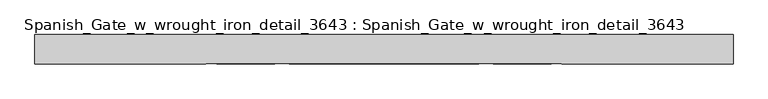
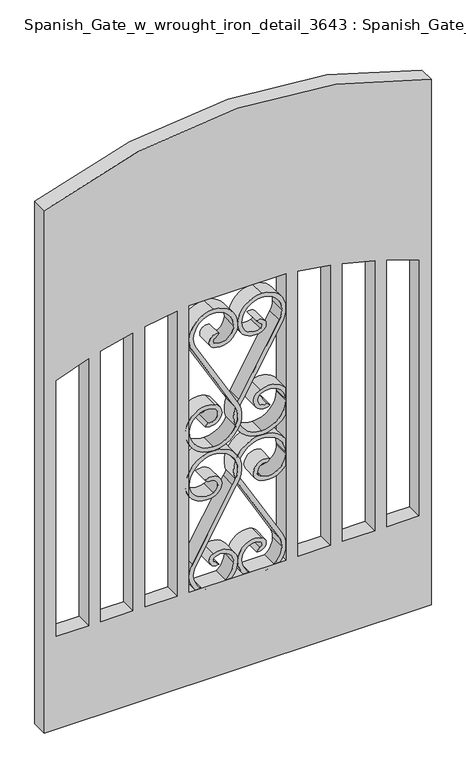
"""IFC4 building model written with IfcOpenShell, lengths in millimetres: proxy geometry, Spanish_Gate_w_wrought_iron_detail_3643 : Spanish_Gate_w_wrought_iron_detail_3643."""

from ifc_helpers import new_model, si_unit, point, frame, frame_2d, origin, place, context, project, spatial, polyline, circle_curve, trimmed, segment, composite_curve, outline, extrude, source, transform, mapped, element, save


def spanish_gate_w_wrought_iron_detail_3643_spanish_gate_w_2ba93c97(model_context):
    return source(origin(), model_context, "Body", "SweptSolid", [
        extrude(outline(composite_curve([segment(polyline([(-271.0336622, 609.6), (1477.5257324, 609.6)]), True, "CONTINUOUS"), segment(trimmed(circle_curve(frame_2d((13.3799195, 11.1413161)), 1581.7318856), [point((1477.5257324, 609.6))], [point((1468.218734, -609.6))], False, "CARTESIAN"), True, "CONTINUOUS"), segment(polyline([(1468.218734, -609.6), (-271.0336622, -609.6), (-271.0336622, 609.6)]), True, "CONTINUOUS")], self_intersect=False), holes=[composite_curve([segment(polyline([(38.1, -469.9), (38.1, -571.5), (888.7988681, -571.5)]), True, "CONTINUOUS"), segment(trimmed(circle_curve(frame_2d((-545.1422563, 0.0)), 1543.6318856), [point((888.7988681, -571.5))], [point((925.2295974, -469.9))], True, "CARTESIAN"), True, "CONTINUOUS"), segment(polyline([(925.2295974, -469.9), (38.1, -469.9)]), True, "CONTINUOUS")], self_intersect=False), composite_curve([segment(polyline([(38.1, 571.5), (38.1, 469.9), (925.2295974, 469.9)]), True, "CONTINUOUS"), segment(trimmed(circle_curve(frame_2d((-545.1422563, 0.0)), 1543.6318856), [point((925.2295974, 469.9))], [point((888.7988681, 571.5))], True, "CARTESIAN"), True, "CONTINUOUS"), segment(polyline([(888.7988681, 571.5), (38.1, 571.5)]), True, "CONTINUOUS")], self_intersect=False), composite_curve([segment(polyline([(38.1, -431.8), (936.8658942, -431.8)]), True, "CONTINUOUS"), segment(trimmed(circle_curve(frame_2d((-545.1422563, 0.0)), 1543.6318856), [point((936.8658942, -431.8))], [point((962.7593845, -330.2))], True, "CARTESIAN"), True, "CONTINUOUS"), segment(polyline([(962.7593845, -330.2), (38.1, -330.2), (38.1, -431.8)]), True, "CONTINUOUS")], self_intersect=False), composite_curve([segment(polyline([(936.8658942, 431.8), (38.1, 431.8), (38.1, 330.2), (962.7593845, 330.2)]), True, "CONTINUOUS"), segment(trimmed(circle_curve(frame_2d((-545.1422563, 0.0)), 1543.6318856), [point((962.7593845, 330.2))], [point((936.8658942, 431.8))], True, "CARTESIAN"), True, "CONTINUOUS")], self_intersect=False), composite_curve([segment(polyline([(38.1, -292.1), (970.6007919, -292.1)]), True, "CONTINUOUS"), segment(trimmed(circle_curve(frame_2d((-545.1422563, 0.0)), 1543.6318856), [point((970.6007919, -292.1))], [point((986.6897019, -190.5))], True, "CARTESIAN"), True, "CONTINUOUS"), segment(polyline([(986.6897019, -190.5), (38.1, -190.5), (38.1, -292.1)]), True, "CONTINUOUS")], self_intersect=False), composite_curve([segment(polyline([(970.6007919, 292.1), (38.1, 292.1), (38.1, 190.5), (986.6897019, 190.5)]), True, "CONTINUOUS"), segment(trimmed(circle_curve(frame_2d((-545.1422563, 0.0)), 1543.6318856), [point((986.6897019, 190.5))], [point((970.6007919, 292.1))], True, "CARTESIAN"), True, "CONTINUOUS")], self_intersect=False), composite_curve([segment(polyline([(38.1, 152.4), (38.1, -152.4), (990.9481181, -152.4)]), True, "CONTINUOUS"), segment(trimmed(circle_curve(frame_2d((-545.1422563, 0.0)), 1543.6318856), [point((990.9481181, -152.4))], [point((990.9481181, 152.4))], True, "CARTESIAN"), True, "CONTINUOUS"), segment(polyline([(990.9481181, 152.4), (38.1, 152.4)]), True, "CONTINUOUS")], self_intersect=False)]), frame((0.0, -50.8, 0.0), z_axis=(0.0, 1.0, 0.0), x_axis=(0.0, 0.0, 1.0)), (0.0, 0.0, 1.0), 50.8),
        extrude(outline(composite_curve([segment(trimmed(circle_curve(frame_2d((876.3, -76.2)), 76.2), [point((876.3, 0.0))], [point((952.5, -76.2))], False, "CARTESIAN"), True, "CONTINUOUS"), segment(trimmed(circle_curve(frame_2d((876.3, -76.2)), 76.2), [point((952.5, -76.2))], [point((876.3, -152.4))], False, "CARTESIAN"), True, "CONTINUOUS"), segment(trimmed(circle_curve(frame_2d((876.3, -76.2)), 76.2), [point((876.3, -152.4))], [point((838.35215, -142.278746))], False, "CARTESIAN"), True, "CONTINUOUS"), segment(polyline([(838.35215, -142.278746), (617.4795877, -15.4355571)]), True, "CONTINUOUS"), segment(trimmed(circle_curve(frame_2d((571.5, -76.2)), 76.2), [point((617.4795877, -15.4355571))], [point((495.3, -76.2))], True, "CARTESIAN"), True, "CONTINUOUS"), segment(trimmed(circle_curve(frame_2d((571.5, -76.2)), 76.2), [point((495.3, -76.2))], [point((571.5, -152.4))], True, "CARTESIAN"), True, "CONTINUOUS"), segment(trimmed(circle_curve(frame_2d((571.5, -97.3666667)), 55.0333333), [point((571.5, -152.4))], [point((622.3, -76.2))], True, "CARTESIAN"), True, "CONTINUOUS"), segment(trimmed(circle_curve(frame_2d((601.7846154, -84.7480769)), 22.225), [point((622.3, -76.2))], [point((581.2692308, -93.2961538))], True, "CARTESIAN"), True, "CONTINUOUS"), segment(polyline([(581.2692308, -93.2961538), (571.8411264, -102.7242582)]), True, "CONTINUOUS"), segment(trimmed(circle_curve(frame_2d((601.7846154, -84.7480769)), 34.925), [point((571.8411264, -102.7242582))], [point((634.0230769, -71.3153846))], False, "CARTESIAN"), True, "CONTINUOUS"), segment(trimmed(circle_curve(frame_2d((571.5, -97.3666667)), 67.7333333), [point((634.0230769, -71.3153846))], [point((571.5, -165.1))], False, "CARTESIAN"), True, "CONTINUOUS"), segment(trimmed(circle_curve(frame_2d((571.5, -76.2)), 88.9), [point((571.5, -165.1))], [point((482.6, -76.2))], False, "CARTESIAN"), True, "CONTINUOUS"), segment(trimmed(circle_curve(frame_2d((571.5, -76.2)), 88.9), [point((482.6, -76.2))], [point((624.474622, -4.8074274))], False, "CARTESIAN"), True, "CONTINUOUS"), segment(polyline([(624.474622, -4.8074274), (844.6767917, -131.2656217)]), True, "CONTINUOUS"), segment(trimmed(circle_curve(frame_2d((876.3, -76.2)), 63.5), [point((844.6767917, -131.2656217))], [point((876.3, -139.7))], True, "CARTESIAN"), True, "CONTINUOUS"), segment(trimmed(circle_curve(frame_2d((876.3, -76.2)), 63.5), [point((876.3, -139.7))], [point((939.8, -76.2))], True, "CARTESIAN"), True, "CONTINUOUS"), segment(trimmed(circle_curve(frame_2d((876.3, -76.2)), 63.5), [point((939.8, -76.2))], [point((876.3, -12.7))], True, "CARTESIAN"), True, "CONTINUOUS"), segment(trimmed(circle_curve(frame_2d((876.3, -55.0333333)), 42.3333333), [point((876.3, -12.7))], [point((837.2230769, -71.3153846))], True, "CARTESIAN"), True, "CONTINUOUS"), segment(trimmed(circle_curve(frame_2d((846.0153846, -67.6519231)), 9.525), [point((837.2230769, -71.3153846))], [point((855.0907531, -70.5438623))], True, "CARTESIAN"), True, "CONTINUOUS"), segment(polyline([(855.0907531, -70.5438623), (866.5307692, -59.1038462)]), True, "CONTINUOUS"), segment(trimmed(circle_curve(frame_2d((846.0153846, -67.6519231)), 22.225), [point((866.5307692, -59.1038462))], [point((825.5, -76.2))], False, "CARTESIAN"), True, "CONTINUOUS"), segment(trimmed(circle_curve(frame_2d((876.3, -55.0333333)), 55.0333333), [point((825.5, -76.2))], [point((876.3, 0.0))], False, "CARTESIAN"), True, "CONTINUOUS")], self_intersect=False)), frame((0.0, -50.8, 0.0), z_axis=(0.0, 1.0, 0.0), x_axis=(0.0, 0.0, 1.0)), (0.0, 0.0, 1.0), 50.8),
        extrude(outline(composite_curve([segment(trimmed(circle_curve(frame_2d((876.3, 55.0333333)), 55.0333333), [point((876.3, 0.0))], [point((825.5, 76.2))], False, "CARTESIAN"), True, "CONTINUOUS"), segment(trimmed(circle_curve(frame_2d((846.0153846, 67.6519231)), 22.225), [point((825.5, 76.2))], [point((866.5307692, 59.1038462))], False, "CARTESIAN"), True, "CONTINUOUS"), segment(polyline([(866.5307692, 59.1038462), (855.0907531, 70.5438623)]), True, "CONTINUOUS"), segment(trimmed(circle_curve(frame_2d((846.0153846, 67.6519231)), 9.525), [point((855.0907531, 70.5438623))], [point((837.2230769, 71.3153846))], True, "CARTESIAN"), True, "CONTINUOUS"), segment(trimmed(circle_curve(frame_2d((876.3, 55.0333333)), 42.3333333), [point((837.2230769, 71.3153846))], [point((876.3, 12.7))], True, "CARTESIAN"), True, "CONTINUOUS"), segment(trimmed(circle_curve(frame_2d((876.3, 76.2)), 63.5), [point((876.3, 12.7))], [point((939.8, 76.2))], True, "CARTESIAN"), True, "CONTINUOUS"), segment(trimmed(circle_curve(frame_2d((876.3, 76.2)), 63.5), [point((939.8, 76.2))], [point((876.3, 139.7))], True, "CARTESIAN"), True, "CONTINUOUS"), segment(trimmed(circle_curve(frame_2d((876.3, 76.2)), 63.5), [point((876.3, 139.7))], [point((844.6767917, 131.2656217))], True, "CARTESIAN"), True, "CONTINUOUS"), segment(polyline([(844.6767917, 131.2656217), (624.474622, 4.8074274)]), True, "CONTINUOUS"), segment(trimmed(circle_curve(frame_2d((571.5, 76.2)), 88.9), [point((624.474622, 4.8074274))], [point((482.6, 76.2))], False, "CARTESIAN"), True, "CONTINUOUS"), segment(trimmed(circle_curve(frame_2d((571.5, 76.2)), 88.9), [point((482.6, 76.2))], [point((571.5, 165.1))], False, "CARTESIAN"), True, "CONTINUOUS"), segment(trimmed(circle_curve(frame_2d((571.5, 97.3666667)), 67.7333333), [point((571.5, 165.1))], [point((634.0230769, 71.3153846))], False, "CARTESIAN"), True, "CONTINUOUS"), segment(trimmed(circle_curve(frame_2d((601.7846154, 84.7480769)), 34.925), [point((634.0230769, 71.3153846))], [point((571.8411264, 102.7242582))], False, "CARTESIAN"), True, "CONTINUOUS"), segment(polyline([(571.8411264, 102.7242582), (581.2692308, 93.2961538)]), True, "CONTINUOUS"), segment(trimmed(circle_curve(frame_2d((601.7846154, 84.7480769)), 22.225), [point((581.2692308, 93.2961538))], [point((622.3, 76.2))], True, "CARTESIAN"), True, "CONTINUOUS"), segment(trimmed(circle_curve(frame_2d((571.5, 97.3666667)), 55.0333333), [point((622.3, 76.2))], [point((571.5, 152.4))], True, "CARTESIAN"), True, "CONTINUOUS"), segment(trimmed(circle_curve(frame_2d((571.5, 76.2)), 76.2), [point((571.5, 152.4))], [point((495.3, 76.2))], True, "CARTESIAN"), True, "CONTINUOUS"), segment(trimmed(circle_curve(frame_2d((571.5, 76.2)), 76.2), [point((495.3, 76.2))], [point((617.4795877, 15.4355571))], True, "CARTESIAN"), True, "CONTINUOUS"), segment(polyline([(617.4795877, 15.4355571), (838.35215, 142.278746)]), True, "CONTINUOUS"), segment(trimmed(circle_curve(frame_2d((876.3, 76.2)), 76.2), [point((838.35215, 142.278746))], [point((876.3, 152.4))], False, "CARTESIAN"), True, "CONTINUOUS"), segment(trimmed(circle_curve(frame_2d((876.3, 76.2)), 76.2), [point((876.3, 152.4))], [point((952.5, 76.2))], False, "CARTESIAN"), True, "CONTINUOUS"), segment(trimmed(circle_curve(frame_2d((876.3, 76.2)), 76.2), [point((952.5, 76.2))], [point((876.3, 0.0))], False, "CARTESIAN"), True, "CONTINUOUS")], self_intersect=False)), frame((0.0, -50.8, 0.0), z_axis=(0.0, 1.0, 0.0), x_axis=(0.0, 0.0, 1.0)), (0.0, 0.0, 1.0), 50.8),
        extrude(outline(composite_curve([segment(trimmed(circle_curve(frame_2d((88.9, -55.0333333)), 55.0333333), [point((88.9, 0.0))], [point((139.7, -76.2))], False, "CARTESIAN"), True, "CONTINUOUS"), segment(trimmed(circle_curve(frame_2d((119.1846154, -67.6519231)), 22.225), [point((139.7, -76.2))], [point((98.6692308, -59.1038462))], False, "CARTESIAN"), True, "CONTINUOUS"), segment(polyline([(98.6692308, -59.1038462), (110.1092469, -70.5438623)]), True, "CONTINUOUS"), segment(trimmed(circle_curve(frame_2d((119.1846154, -67.6519231)), 9.525), [point((110.1092469, -70.5438623))], [point((127.9769231, -71.3153846))], True, "CARTESIAN"), True, "CONTINUOUS"), segment(trimmed(circle_curve(frame_2d((88.9, -55.0333333)), 42.3333333), [point((127.9769231, -71.3153846))], [point((88.9, -12.7))], True, "CARTESIAN"), True, "CONTINUOUS"), segment(trimmed(circle_curve(frame_2d((88.9, -76.2)), 63.5), [point((88.9, -12.7))], [point((25.4, -76.2))], True, "CARTESIAN"), True, "CONTINUOUS"), segment(trimmed(circle_curve(frame_2d((88.9, -76.2)), 63.5), [point((25.4, -76.2))], [point((88.9, -139.7))], True, "CARTESIAN"), True, "CONTINUOUS"), segment(trimmed(circle_curve(frame_2d((88.9, -76.2)), 63.5), [point((88.9, -139.7))], [point((120.5232083, -131.2656217))], True, "CARTESIAN"), True, "CONTINUOUS"), segment(polyline([(120.5232083, -131.2656217), (340.725378, -4.8074274)]), True, "CONTINUOUS"), segment(trimmed(circle_curve(frame_2d((393.7, -76.2)), 88.9), [point((340.725378, -4.8074274))], [point((482.6, -76.2))], False, "CARTESIAN"), True, "CONTINUOUS"), segment(trimmed(circle_curve(frame_2d((393.7, -76.2)), 88.9), [point((482.6, -76.2))], [point((393.7, -165.1))], False, "CARTESIAN"), True, "CONTINUOUS"), segment(trimmed(circle_curve(frame_2d((393.7, -97.3666667)), 67.7333333), [point((393.7, -165.1))], [point((331.1769231, -71.3153846))], False, "CARTESIAN"), True, "CONTINUOUS"), segment(trimmed(circle_curve(frame_2d((363.4153846, -84.7480769)), 34.925), [point((331.1769231, -71.3153846))], [point((393.3588736, -102.7242582))], False, "CARTESIAN"), True, "CONTINUOUS"), segment(polyline([(393.3588736, -102.7242582), (383.9307692, -93.2961538)]), True, "CONTINUOUS"), segment(trimmed(circle_curve(frame_2d((363.4153846, -84.7480769)), 22.225), [point((383.9307692, -93.2961538))], [point((342.9, -76.2))], True, "CARTESIAN"), True, "CONTINUOUS"), segment(trimmed(circle_curve(frame_2d((393.7, -97.3666667)), 55.0333333), [point((342.9, -76.2))], [point((393.7, -152.4))], True, "CARTESIAN"), True, "CONTINUOUS"), segment(trimmed(circle_curve(frame_2d((393.7, -76.2)), 76.2), [point((393.7, -152.4))], [point((469.9, -76.2))], True, "CARTESIAN"), True, "CONTINUOUS"), segment(trimmed(circle_curve(frame_2d((393.7, -76.2)), 76.2), [point((469.9, -76.2))], [point((347.7204123, -15.4355571))], True, "CARTESIAN"), True, "CONTINUOUS"), segment(polyline([(347.7204123, -15.4355571), (126.84785, -142.278746)]), True, "CONTINUOUS"), segment(trimmed(circle_curve(frame_2d((88.9, -76.2)), 76.2), [point((126.84785, -142.278746))], [point((88.9, -152.4))], False, "CARTESIAN"), True, "CONTINUOUS"), segment(trimmed(circle_curve(frame_2d((88.9, -76.2)), 76.2), [point((88.9, -152.4))], [point((12.7, -76.2))], False, "CARTESIAN"), True, "CONTINUOUS"), segment(trimmed(circle_curve(frame_2d((88.9, -76.2)), 76.2), [point((12.7, -76.2))], [point((88.9, 0.0))], False, "CARTESIAN"), True, "CONTINUOUS")], self_intersect=False)), frame((0.0, -50.8, 0.0), z_axis=(0.0, 1.0, 0.0), x_axis=(0.0, 0.0, 1.0)), (0.0, 0.0, 1.0), 50.8),
        extrude(outline(composite_curve([segment(trimmed(circle_curve(frame_2d((88.9, 76.2)), 76.2), [point((88.9, 0.0))], [point((12.7, 76.2))], False, "CARTESIAN"), True, "CONTINUOUS"), segment(trimmed(circle_curve(frame_2d((88.9, 76.2)), 76.2), [point((12.7, 76.2))], [point((88.9, 152.4))], False, "CARTESIAN"), True, "CONTINUOUS"), segment(trimmed(circle_curve(frame_2d((88.9, 76.2)), 76.2), [point((88.9, 152.4))], [point((126.84785, 142.278746))], False, "CARTESIAN"), True, "CONTINUOUS"), segment(polyline([(126.84785, 142.278746), (347.7204123, 15.4355571)]), True, "CONTINUOUS"), segment(trimmed(circle_curve(frame_2d((393.7, 76.2)), 76.2), [point((347.7204123, 15.4355571))], [point((469.9, 76.2))], True, "CARTESIAN"), True, "CONTINUOUS"), segment(trimmed(circle_curve(frame_2d((393.7, 76.2)), 76.2), [point((469.9, 76.2))], [point((393.7, 152.4))], True, "CARTESIAN"), True, "CONTINUOUS"), segment(trimmed(circle_curve(frame_2d((393.7, 97.3666667)), 55.0333333), [point((393.7, 152.4))], [point((342.9, 76.2))], True, "CARTESIAN"), True, "CONTINUOUS"), segment(trimmed(circle_curve(frame_2d((363.4153846, 84.7480769)), 22.225), [point((342.9, 76.2))], [point((383.9307692, 93.2961538))], True, "CARTESIAN"), True, "CONTINUOUS"), segment(polyline([(383.9307692, 93.2961538), (393.3588736, 102.7242582)]), True, "CONTINUOUS"), segment(trimmed(circle_curve(frame_2d((363.4153846, 84.7480769)), 34.925), [point((393.3588736, 102.7242582))], [point((331.1769231, 71.3153846))], False, "CARTESIAN"), True, "CONTINUOUS"), segment(trimmed(circle_curve(frame_2d((393.7, 97.3666667)), 67.7333333), [point((331.1769231, 71.3153846))], [point((393.7, 165.1))], False, "CARTESIAN"), True, "CONTINUOUS"), segment(trimmed(circle_curve(frame_2d((393.7, 76.2)), 88.9), [point((393.7, 165.1))], [point((482.6, 76.2))], False, "CARTESIAN"), True, "CONTINUOUS"), segment(trimmed(circle_curve(frame_2d((393.7, 76.2)), 88.9), [point((482.6, 76.2))], [point((340.725378, 4.8074274))], False, "CARTESIAN"), True, "CONTINUOUS"), segment(polyline([(340.725378, 4.8074274), (120.5232083, 131.2656217)]), True, "CONTINUOUS"), segment(trimmed(circle_curve(frame_2d((88.9, 76.2)), 63.5), [point((120.5232083, 131.2656217))], [point((88.9, 139.7))], True, "CARTESIAN"), True, "CONTINUOUS"), segment(trimmed(circle_curve(frame_2d((88.9, 76.2)), 63.5), [point((88.9, 139.7))], [point((25.4, 76.2))], True, "CARTESIAN"), True, "CONTINUOUS"), segment(trimmed(circle_curve(frame_2d((88.9, 76.2)), 63.5), [point((25.4, 76.2))], [point((88.9, 12.7))], True, "CARTESIAN"), True, "CONTINUOUS"), segment(trimmed(circle_curve(frame_2d((88.9, 55.0333333)), 42.3333333), [point((88.9, 12.7))], [point((127.9769231, 71.3153846))], True, "CARTESIAN"), True, "CONTINUOUS"), segment(trimmed(circle_curve(frame_2d((119.1846154, 67.6519231)), 9.525), [point((127.9769231, 71.3153846))], [point((110.1092469, 70.5438623))], True, "CARTESIAN"), True, "CONTINUOUS"), segment(polyline([(110.1092469, 70.5438623), (98.6692308, 59.1038462)]), True, "CONTINUOUS"), segment(trimmed(circle_curve(frame_2d((119.1846154, 67.6519231)), 22.225), [point((98.6692308, 59.1038462))], [point((139.7, 76.2))], False, "CARTESIAN"), True, "CONTINUOUS"), segment(trimmed(circle_curve(frame_2d((88.9, 55.0333333)), 55.0333333), [point((139.7, 76.2))], [point((88.9, 0.0))], False, "CARTESIAN"), True, "CONTINUOUS")], self_intersect=False)), frame((0.0, -50.8, 0.0), z_axis=(0.0, 1.0, 0.0), x_axis=(0.0, 0.0, 1.0)), (0.0, 0.0, 1.0), 50.8),
    ])


if __name__ == "__main__":
    model = new_model("IFC4")
    model_context = context("Model", 3, world=origin())
    ifc_project = project(units=[si_unit("LENGTHUNIT", "METRE", prefix="MILLI")], contexts=[model_context])
    site = spatial("IfcSite", under=ifc_project)
    building = spatial("IfcBuilding", under=site)
    placement = place(None, origin())
    spanish_gate_w_wrought_iron_detail_3643_spanish_gate_w_shape = spanish_gate_w_wrought_iron_detail_3643_spanish_gate_w_2ba93c97(model_context)
    element("IfcBuildingElementProxy", 1, Name="Spanish_Gate_w_wrought_iron_detail_3643 : Spanish_Gate_w_wrought_iron_detail_3643", ObjectType="Spanish_Gate_w_wrought_iron_detail_3643 : Spanish_Gate_w_wrought_iron_detail_3643", at=placement, inside=building, context=model_context, shape_type="MappedRepresentation", body=[
        mapped(spanish_gate_w_wrought_iron_detail_3643_spanish_gate_w_shape, transform((0.0, 0.0, 0.0), x_axis=(1.0, 0.0, 0.0), y_axis=(0.0, 1.0, 0.0), z_axis=(0.0, 0.0, 1.0))),
    ])
    save(model, "model.ifc")

# Revit data of these elements
# Type "Spanish_Gate_w_wrought_iron_detail_3643 : Spanish_Gate_w_wrought_iron_detail_3643"
#   Default Elevation = 0
# Element 1 (IfcBuildingElementProxy, "Spanish_Gate_w_wrought_iron_detail_3643 : Spanish_Gate_w_wrought_iron_detail_3643")
#   Materials on its faces: "iron"
# Materials
#   "iron": colour RGB 49 49 49, transparency 0
